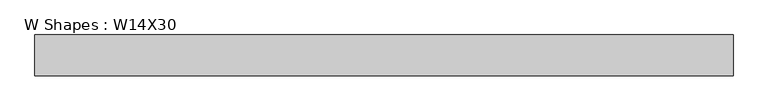
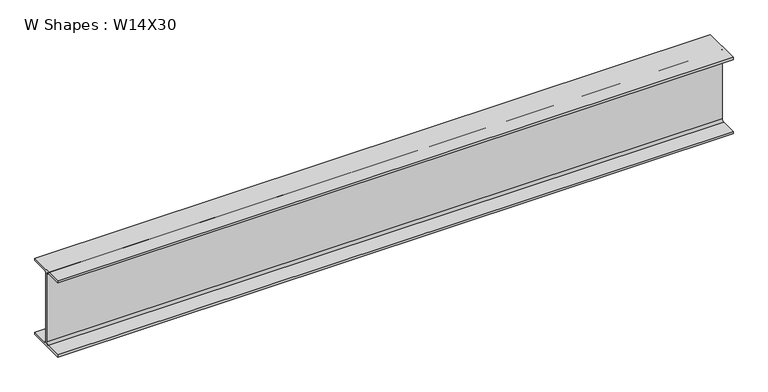
"""IFC4 building model written with IfcOpenShell, lengths in millimetres: beam geometry, W Shapes : W14X30."""

from ifc_helpers import new_model, si_unit, point, frame, frame_2d, origin, place, context, project, spatial, polyline, circle_curve, trimmed, segment, composite_curve, outline, extrude, source, transform, mapped, element, save


def w_shapes_w14x30_a113fbeb(model_context):
    return source(origin(), model_context, "Body", "SweptSolid", [
        extrude(outline(composite_curve([segment(polyline([(85.471, -165.481), (85.471, -175.26), (-85.471, -175.26), (-85.471, -165.481), (-13.589, -165.481)]), True, "CONTINUOUS"), segment(trimmed(circle_curve(frame_2d((-13.589, -155.321)), 10.16), [point((-13.589, -165.481))], [point((-3.429, -155.321))], True, "CARTESIAN"), True, "CONTINUOUS"), segment(polyline([(-3.429, -155.321), (-3.429, 155.321)]), True, "CONTINUOUS"), segment(trimmed(circle_curve(frame_2d((-13.589, 155.321)), 10.16), [point((-3.429, 155.321))], [point((-13.589, 165.481))], True, "CARTESIAN"), True, "CONTINUOUS"), segment(polyline([(-13.589, 165.481), (-85.471, 165.481), (-85.471, 175.26), (85.471, 175.26), (85.471, 165.481), (13.589, 165.481)]), True, "CONTINUOUS"), segment(trimmed(circle_curve(frame_2d((13.589, 155.321)), 10.16), [point((13.589, 165.481))], [point((3.429, 155.321))], True, "CARTESIAN"), True, "CONTINUOUS"), segment(polyline([(3.429, 155.321), (3.429, -155.321)]), True, "CONTINUOUS"), segment(trimmed(circle_curve(frame_2d((13.589, -155.321)), 10.16), [point((3.429, -155.321))], [point((13.589, -165.481))], True, "CARTESIAN"), True, "CONTINUOUS"), segment(polyline([(13.589, -165.481), (85.471, -165.481)]), True, "CONTINUOUS")], self_intersect=False)), frame((-1386.8106892, 0.0, 0.0), z_axis=(1.0, 0.0, 0.0), x_axis=(0.0, 1.0, 0.0)), (0.0, 0.0, 1.0), 2933.2566267),
    ])


if __name__ == "__main__":
    model = new_model("IFC4")
    model_context = context("Model", 3, world=origin())
    ifc_project = project(units=[si_unit("LENGTHUNIT", "METRE", prefix="MILLI")], contexts=[model_context])
    site = spatial("IfcSite", under=ifc_project)
    building = spatial("IfcBuilding", under=site)
    placement = place(None, origin())
    w_shapes_w14x30_shape = w_shapes_w14x30_a113fbeb(model_context)
    element("IfcBeam", 1, ObjectType="W Shapes : W14X30", at=placement, inside=building, context=model_context, shape_type="MappedRepresentation", body=[
        mapped(w_shapes_w14x30_shape, transform((0.0, 0.0, 0.0), x_axis=(1.0, 0.0, 0.0), y_axis=(0.0, 1.0, 0.0), z_axis=(0.0, 0.0, 1.0))),
    ])
    save(model, "model.ifc")

# Revit data of these elements
# Type "W Shapes : W14X30"
#   Section Name Key = "W14X30"
#   Width = 6.730"
#   Web Thickness = 0.270"
#   Web Fillet = 0.400"
#   Warping Constant = 887.00 in⁶
#   Torsional Moment of Inertia = 0.38 in⁴
#   Section Area = 8.85 in²
#   Plastic Modulus weak axis = 8.99 in³
#   Plastic Modulus strong axis = 47.30 in³
#   Perimeter = 4.441 ft²/ft
#   Nominal Weight = 30.00 lbf/ft
#   Moment of Inertia weak axis = 19.60 in⁴
#   Moment of Inertia strong axis = 291.00 in⁴
#   Height = 13.800"
#   Flange Thickness = 0.385"
#   Elastic Modulus weak axis = 5.82 in³
#   Elastic Modulus strong axis = 42.00 in³
#   Clear Web Height = 0' - 11 5/8"
#   Centroid Vertical = 6.900"
#   Centroid Horizontal = 3.365"
#   Bolt Spacing = 0' - 3 1/2"
#   Length [instance default] = 1524 mm
#   Structural Material [instance default] = Steel ASTM A992
#   Principal Axes Angle = 0
# Element 1 (IfcBeam, "W Shapes : W14X30")
#   Length = 3871.876 mm
#   Materials on its faces: "Steel ASTM A992"
# Materials
#   "Steel ASTM A992": class "Metal", colour RGB 199 199 199, transparency 0, Description = "Structural steel 50ksi", Cost = 0
